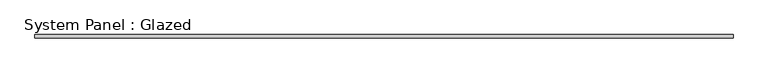
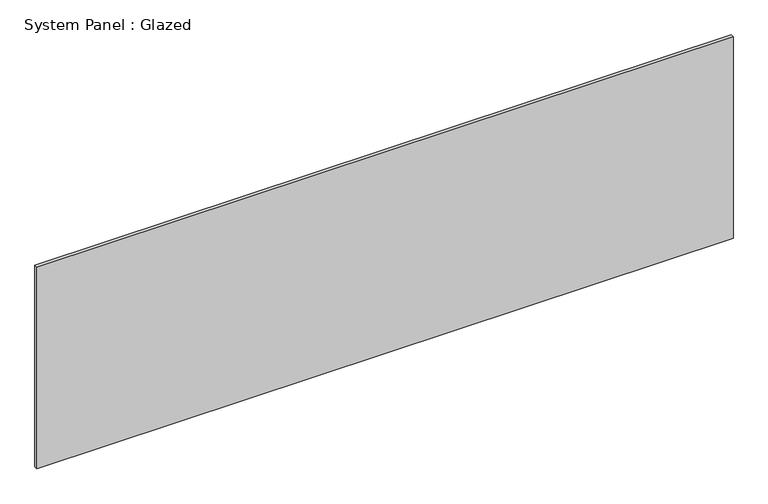
"""IFC4 building model written with IfcOpenShell, lengths in millimetres: plate geometry, System Panel : Glazed."""

from ifc_helpers import new_model, si_unit, origin, origin_with_axes, place, context, project, spatial, polyline, outline, extrude, source, transform, mapped, element, save


def system_panel_glazed_e45de85a(model_context):
    return source(origin(), model_context, "Body", "SweptSolid", [
        extrude(outline(polyline([(2491.2842472, 19.05), (-2491.2842472, 19.05), (-2491.2842472, 44.45), (2491.2842472, 44.45), (2491.2842472, 19.05)])), origin_with_axes(), (0.0, 0.0, 1.0), 1524.0),
    ])


if __name__ == "__main__":
    model = new_model("IFC4")
    model_context = context("Model", 3, world=origin())
    ifc_project = project(units=[si_unit("LENGTHUNIT", "METRE", prefix="MILLI")], contexts=[model_context])
    site = spatial("IfcSite", under=ifc_project)
    building = spatial("IfcBuilding", under=site)
    placement = place(None, origin())
    system_panel_glazed_shape = system_panel_glazed_e45de85a(model_context)
    element("IfcPlate", 1, ObjectType="System Panel : Glazed", at=placement, inside=building, context=model_context, shape_type="MappedRepresentation", body=[
        mapped(system_panel_glazed_shape, transform((0.0, 0.0, 0.0), x_axis=(1.0, 0.0, 0.0), y_axis=(0.0, 1.0, 0.0), z_axis=(0.0, 0.0, 1.0))),
    ])
    save(model, "model.ifc")

# Revit data of these elements
# Type "System Panel : Glazed"
#   Construction Type Id = "GSP4R"
#   Analytic Construction = "1/8 in Pilkington single glazing"
#   Visual Light Transmittance = 0.9
#   Solar Heat Gain Coefficient = 0.86
#   Heat Transfer Coefficient (U) = 1.18115 BTU/(h·ft²·°F)
# Element 1 (IfcPlate, "System Panel : Glazed")
#   Materials on its faces: "Glass"
# Materials
#   "Glass": class "Glass", colour RGB 0 128 192, transparency 0.75, Description = "Soda Lime Glass", Cost = 0
